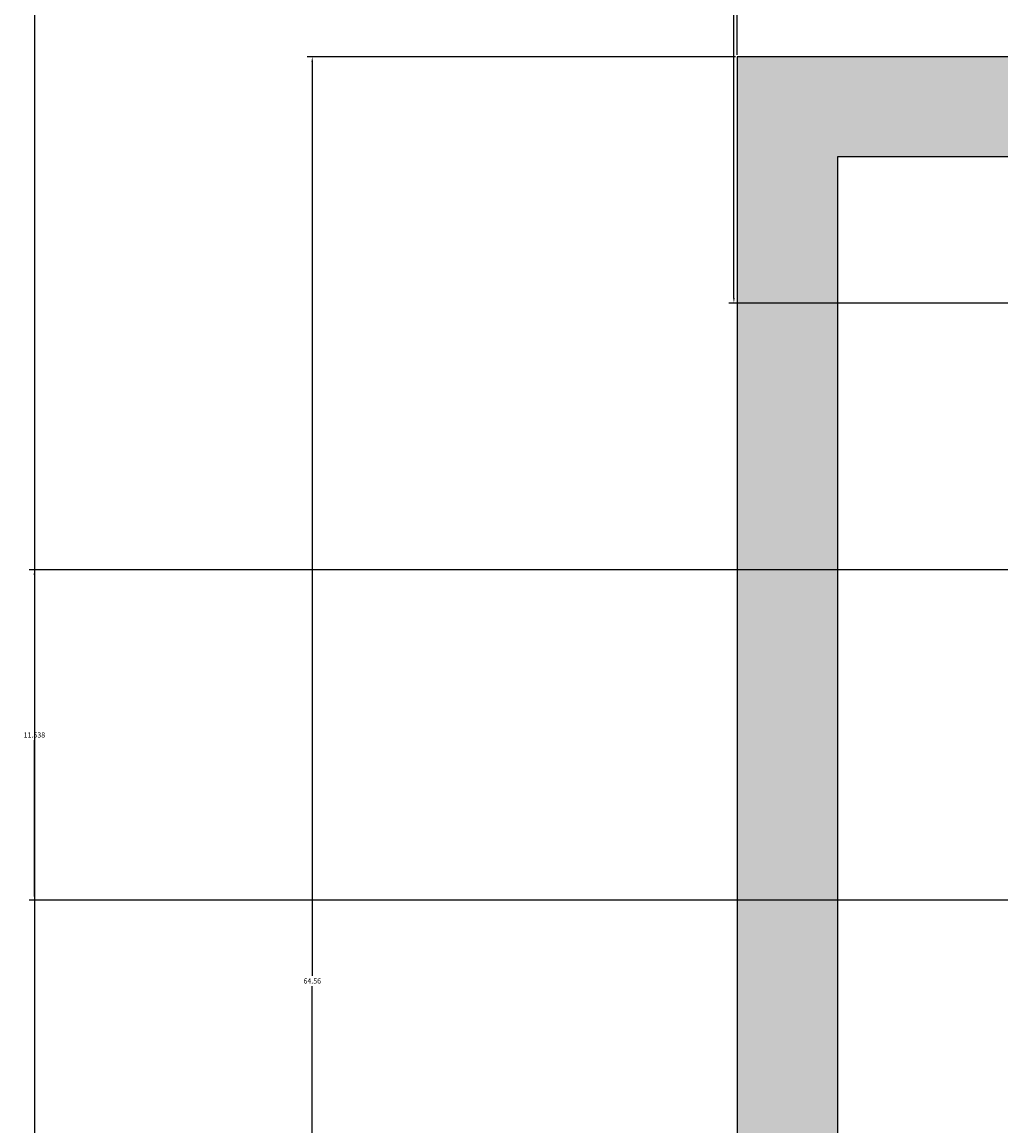
# Model space of a CAD drawing. Units: millimetres. Extents: x -11 to 280, y -4 to 208.
# Tile 7 of 55: x -11 to 24, y 125 to 164. Entities that reach past the tile are written whole.
import ezdxf

# ---------------------------------------------------------------- set-up
doc = ezdxf.new("R2010")
doc.units = ezdxf.units.MM
doc.layers.add('M-DIMS', color=2, linetype='Continuous', lineweight=18)
doc.layers.add('M-HYDR-RETN', color=7, linetype='Continuous', lineweight=25)
doc.layers.add('M-HYDR-RETN-PATT', color=114, linetype='Continuous', lineweight=13, true_color=0x139b48)
doc.styles.get("Standard").update_dxf_attribs({"font": 'arial.ttf'})
doc.dimstyles.get("Standard").update_dxf_attribs({"dimtxt": 0.18, "dimasz": 0.18, "dimexe": 0.18, "dimexo": 0.0625, "dimgap": 0.09, "dimtad": 0, "dimtih": 1, "dimtoh": 1, "dimdec": 4, "dimzin": 0, "dimdsep": 46, "dimtxsty": 'Standard', "dimcen": 0.09, "dimadec": 0, "dimazin": 0, "dimtfac": 1, "dimtdec": 4, "dimtofl": 0, "dimtmove": 0, "dimatfit": 3, "dimfxl": 1, "dimtolj": 1, "dimtzin": 0, "dimarcsym": 0})

# ---------------------------------------------------------------- blocks, each defined once
blk = doc.blocks.new('*D5')
at = {"layer": 'Defpoints', "color": 0, "transparency": 16777216}
for p in [(24.759, 192.645), (-10.087, 11.435), (261.686, 11.435)]:
    blk.add_point(p, dxfattribs=at)
at = {"layer": 'M-DIMS', "color": 0, "lineweight": -2, "transparency": 16777216}
for p, q in [((24.696, 192.645), (-10.267, 192.645)), ((-10.087, 192.465), (-10.087, 102.222)), ((-10.087, 11.615), (-10.087, 101.858)), ((261.624, 11.435), (-10.267, 11.435))]:
    blk.add_line(p, q, dxfattribs=at)
at = {"layer": 'M-DIMS', "color": 0, "transparency": 16777216}
for points in [[(-10.117, 192.465), (-10.057, 192.465), (-10.087, 192.645)], [(-10.117, 11.615), (-10.057, 11.615), (-10.087, 11.435)]]:
    blk.add_solid(points, dxfattribs=at)
at = {"layer": 'M-DIMS', "color": 0, "transparency": 16777216, "insert": (-10.087, 102.04), "char_height": 0.18, "attachment_point": 5}
blk.add_mtext('\\A1;181.2', dxfattribs=at)
blk = doc.blocks.new('*D7')
at = {"layer": 'Defpoints', "color": 0, "transparency": 16777216}
for p in [(-0.38, 162.581), (14.47, 162.581), (14.47, 98.021)]:
    blk.add_point(p, dxfattribs=at)
at = {"layer": 'M-DIMS', "color": 0, "lineweight": -2, "transparency": 16777216}
for p, q in [((14.408, 162.581), (-0.56, 162.581)), ((-0.38, 162.401), (-0.38, 130.483)), ((-0.38, 98.201), (-0.38, 130.119)), ((14.408, 98.021), (-0.56, 98.021))]:
    blk.add_line(p, q, dxfattribs=at)
at = {"layer": 'M-DIMS', "color": 0, "transparency": 16777216}
for points in [[(-0.41, 162.401), (-0.35, 162.401), (-0.38, 162.581)], [(-0.41, 98.201), (-0.35, 98.201), (-0.38, 98.021)]]:
    blk.add_solid(points, dxfattribs=at)
at = {"layer": 'M-DIMS', "color": 0, "transparency": 16777216, "insert": (-0.38, 130.301), "char_height": 0.18, "attachment_point": 5}
blk.add_mtext('\\A1;64.56', dxfattribs=at)
blk = doc.blocks.new('*D8')
at = {"layer": 'Defpoints', "color": 0, "transparency": 16777216}
for p in [(29.201, 177.431), (14.47, 162.581), (29.201, 162.581)]:
    blk.add_point(p, dxfattribs=at)
at = {"layer": 'M-DIMS', "color": 0, "lineweight": -2, "transparency": 16777216}
for p, q in [((14.47, 162.644), (14.47, 177.611)), ((14.65, 177.431), (21.451, 177.431)), ((29.021, 177.431), (22.221, 177.431)), ((29.201, 162.644), (29.201, 177.611))]:
    blk.add_line(p, q, dxfattribs=at)
at = {"layer": 'M-DIMS', "color": 0, "transparency": 16777216}
for points in [[(14.65, 177.461), (14.65, 177.401), (14.47, 177.431)], [(29.021, 177.461), (29.021, 177.401), (29.201, 177.431)]]:
    blk.add_solid(points, dxfattribs=at)
at = {"layer": 'M-DIMS', "color": 0, "transparency": 16777216, "insert": (21.836, 177.431), "char_height": 0.18, "attachment_point": 5}
blk.add_mtext('\\A1;14.73', dxfattribs=at)
blk = doc.blocks.new('*D14')
at = {"layer": 'Defpoints', "color": 0, "transparency": 16777216}
for p in [(-10.087, 144.661), (205.531, 144.661), (226.511, 133.123)]:
    blk.add_point(p, dxfattribs=at)
at = {"layer": 'M-DIMS', "color": 0, "lineweight": -2, "transparency": 16777216}
for p, q in [((205.469, 144.661), (-10.267, 144.661)), ((-10.087, 144.481), (-10.087, 139.074)), ((-10.087, 133.303), (-10.087, 138.71)), ((226.448, 133.123), (-10.267, 133.123))]:
    blk.add_line(p, q, dxfattribs=at)
at = {"layer": 'M-DIMS', "color": 0, "transparency": 16777216}
for points in [[(-10.117, 144.481), (-10.057, 144.481), (-10.087, 144.661)], [(-10.117, 133.303), (-10.057, 133.303), (-10.087, 133.123)]]:
    blk.add_solid(points, dxfattribs=at)
at = {"layer": 'M-DIMS', "color": 0, "transparency": 16777216, "insert": (-10.087, 138.892), "char_height": 0.18, "attachment_point": 5}
blk.add_mtext('\\A1;11.538', dxfattribs=at)
blk = doc.blocks.new('*D24')
at = {"layer": 'Defpoints', "color": 0, "transparency": 16777216}
for p in [(14.351, 179.241), (29.201, 179.241), (29.201, 153.977)]:
    blk.add_point(p, dxfattribs=at)
at = {"layer": 'M-DIMS', "color": 0, "lineweight": -2, "transparency": 16777216}
for p, q in [((29.139, 179.241), (14.171, 179.241)), ((14.351, 179.061), (14.351, 166.791)), ((14.351, 154.157), (14.351, 166.427)), ((29.139, 153.977), (14.171, 153.977))]:
    blk.add_line(p, q, dxfattribs=at)
at = {"layer": 'M-DIMS', "color": 0, "transparency": 16777216}
for points in [[(14.321, 179.061), (14.381, 179.061), (14.351, 179.241)], [(14.321, 154.157), (14.381, 154.157), (14.351, 153.977)]]:
    blk.add_solid(points, dxfattribs=at)
at = {"layer": 'M-DIMS', "color": 0, "transparency": 16777216, "insert": (14.351, 166.609), "char_height": 0.18, "attachment_point": 5}
blk.add_mtext('\\A1;25.264', dxfattribs=at)

msp = doc.modelspace()

# ---------------------------------------------------------------- hatches: boundary and pattern name
at = {"layer": 'M-HYDR-RETN-PATT'}
h = msp.add_hatch(color=256, dxfattribs=at)
h.set_gradient(color1=(19, 155, 72), color2=(19, 155, 72), tint=1)
h.paths.add_polyline_path([(17.9701, 159.0814), (29.2015, 159.0814), (29.2015, 162.5814), (14.4701, 162.5814), (14.4701, 98.0213), (17.9701, 98.0213)])
h.paths.add_polyline_path([(17.9701, 84.4261), (14.4701, 84.4261), (14.4701, 54.3099), (156.2446, 54.3099), (156.2446, 57.8099), (17.9701, 57.8099)])
h.paths.add_polyline_path([(120.5137, 74.3991), (17.9701, 74.3991), (17.9701, 70.8991), (120.5137, 70.8991)], flags=17)
h.paths.add_polyline_path([(184.7092, 75.04, 0.4142136), (179.7092, 80.04), (156.2446, 80.04), (156.2446, 57.8099), (156.2446, 54.3099), (156.2446, 43.5991), (159.7446, 43.5991), (159.7446, 57.8099), (159.7446, 76.54), (176.2092, 76.54, -0.4142136), (181.2092, 71.54), (181.2092, 57.8099), (159.7446, 57.8099), (159.7446, 54.3099), (184.7092, 54.3099)])

# ---------------------------------------------------------------- linework, layer by layer
at = {"layer": 'M-HYDR-RETN'}
for p, q in [((29.2015, 162.5814), (14.4701, 162.5814)), ((29.2015, 159.0814), (17.9701, 159.0814))]:
    msp.add_line(p, q, dxfattribs=at)
for points in [[(14.4701, 162.5814), (14.4701, 98.0213)], [(17.9701, 159.0814), (17.9701, 98.0213)]]:
    msp.add_lwpolyline(points, dxfattribs=at)

# ---------------------------------------------------------------- dimensions: what is measured, and where the dimension line sits
at = {"layer": 'M-DIMS'}
for base, p1, p2, override, picture, middle in [((-10.0865, 11.4346), (24.7588, 192.645), (261.6863, 11.4346), {"dimdec": 1, "dimlfac": 1, "dimrnd": 0, "dimzin": 0, "dimdsep": 46, "dimlunit": 2}, '*D5', (-10.0865, 102.0398)), ((14.3515, 179.2412), (29.2015, 153.9768), (29.2015, 179.2412), {"dimdec": 3, "dimlfac": 1, "dimrnd": 0, "dimzin": 0, "dimdsep": 46, "dimlunit": 2}, '*D24', (14.3515, 166.609)), ((-0.3799, 162.5814), (14.4701, 98.0213), (14.4701, 162.5814), {"dimdec": 2, "dimlfac": 1, "dimrnd": 0, "dimzin": 0, "dimdsep": 46, "dimlunit": 2}, '*D7', (-0.3799, 130.3014)), ((-10.0865, 144.6609), (226.5106, 133.1228), (205.5315, 144.6609), {"dimdec": 3, "dimlfac": 1, "dimrnd": 0, "dimzin": 0, "dimdsep": 46, "dimlunit": 2}, '*D14', (-10.0865, 138.8918))]:
    dim = msp.add_linear_dim(base=base, p1=p1, p2=p2, angle=90, dimstyle='Standard', override=override, dxfattribs=at)
    dim.commit()
    dim.dimension.update_dxf_attribs({"geometry": picture, "text_midpoint": middle})
dim = msp.add_linear_dim(base=(29.2015, 177.4314), p1=(14.4701, 162.5814), p2=(29.2015, 162.5814), dimstyle='Standard', override={"dimdec": 2, "dimlfac": 1, "dimrnd": 0, "dimzin": 0, "dimdsep": 46, "dimlunit": 2}, dxfattribs=at)
dim.commit()
dim.dimension.update_dxf_attribs({"geometry": '*D8', "text_midpoint": (21.8358, 177.4314)})

doc.saveas('drawing.dxf')
